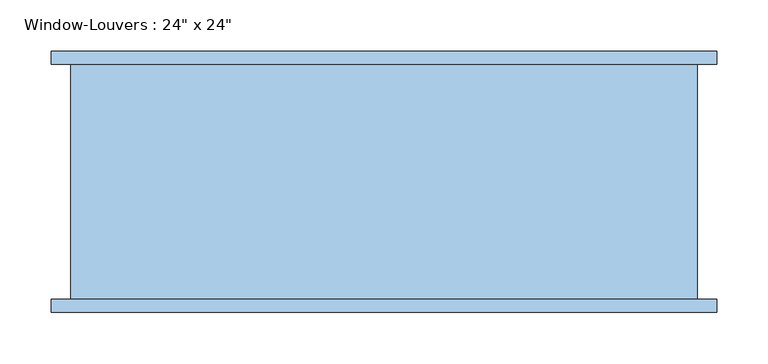
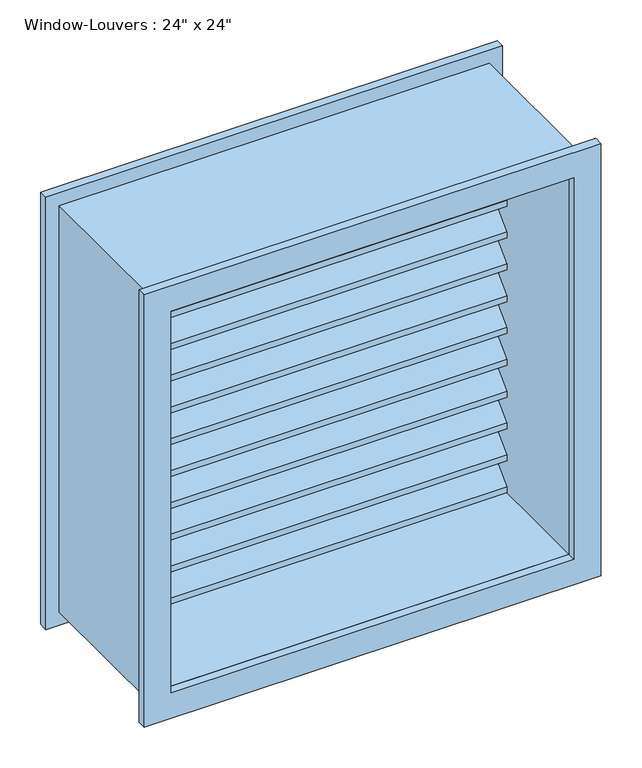
"""IFC4 building model written with IfcOpenShell, lengths in millimetres: window geometry."""

from ifc_helpers import new_model, si_unit, frame, origin, place, context, project, spatial, polyline, outline, extrude, source, transform, mapped, element, save


def window_f2d8fef0(model_context):
    return source(origin(), model_context, "Body", "SweptSolid", [
        extrude(outline(polyline([(107.95, 1419.1754778), (107.95, 1410.1952217), (69.85, 1448.2952217), (31.75, 1410.1952217), (31.75, 1419.1754778), (69.85, 1457.2754778), (107.95, 1419.1754778)])), frame((-285.75, 0.0, 0.0), z_axis=(1.0, 0.0, 0.0), x_axis=(0.0, 1.0, 0.0)), (0.0, 0.0, 1.0), 571.5),
        extrude(outline(polyline([(107.95, 1371.5009557), (107.95, 1362.5206995), (69.85, 1400.6206995), (31.75, 1362.5206995), (31.75, 1371.5009557), (69.85, 1409.6009557), (107.95, 1371.5009557)])), frame((-285.75, 0.0, 0.0), z_axis=(1.0, 0.0, 0.0), x_axis=(0.0, 1.0, 0.0)), (0.0, 0.0, 1.0), 571.5),
        extrude(outline(polyline([(107.95, 1323.8264335), (107.95, 1314.8461774), (69.85, 1352.9461774), (31.75, 1314.8461774), (31.75, 1323.8264335), (69.85, 1361.9264335), (107.95, 1323.8264335)])), frame((-285.75, 0.0, 0.0), z_axis=(1.0, 0.0, 0.0), x_axis=(0.0, 1.0, 0.0)), (0.0, 0.0, 1.0), 571.5),
        extrude(outline(polyline([(107.95, 1276.1519113), (107.95, 1267.1716552), (69.85, 1305.2716552), (31.75, 1267.1716552), (31.75, 1276.1519113), (69.85, 1314.2519113), (107.95, 1276.1519113)])), frame((-285.75, 0.0, 0.0), z_axis=(1.0, 0.0, 0.0), x_axis=(0.0, 1.0, 0.0)), (0.0, 0.0, 1.0), 571.5),
        extrude(outline(polyline([(107.95, 1228.4773891), (107.95, 1219.497133), (69.85, 1257.597133), (31.75, 1219.497133), (31.75, 1228.4773891), (69.85, 1266.5773891), (107.95, 1228.4773891)])), frame((-285.75, 0.0, 0.0), z_axis=(1.0, 0.0, 0.0), x_axis=(0.0, 1.0, 0.0)), (0.0, 0.0, 1.0), 571.5),
        extrude(outline(polyline([(107.95, 1180.802867), (107.95, 1171.8226109), (69.85, 1209.9226109), (31.75, 1171.8226109), (31.75, 1180.802867), (69.85, 1218.902867), (107.95, 1180.802867)])), frame((-285.75, 0.0, 0.0), z_axis=(1.0, 0.0, 0.0), x_axis=(0.0, 1.0, 0.0)), (0.0, 0.0, 1.0), 571.5),
        extrude(outline(polyline([(107.95, 1133.1283448), (107.95, 1124.1480887), (69.85, 1162.2480887), (31.75, 1124.1480887), (31.75, 1133.1283448), (69.85, 1171.2283448), (107.95, 1133.1283448)])), frame((-285.75, 0.0, 0.0), z_axis=(1.0, 0.0, 0.0), x_axis=(0.0, 1.0, 0.0)), (0.0, 0.0, 1.0), 571.5),
        extrude(outline(polyline([(107.95, 1085.4538226), (107.95, 1076.4735665), (69.85, 1114.5735665), (31.75, 1076.4735665), (31.75, 1085.4538226), (69.85, 1123.5538226), (107.95, 1085.4538226)])), frame((-285.75, 0.0, 0.0), z_axis=(1.0, 0.0, 0.0), x_axis=(0.0, 1.0, 0.0)), (0.0, 0.0, 1.0), 571.5),
        extrude(outline(polyline([(107.95, 1037.7793005), (107.95, 1028.7990443), (69.85, 1066.8990443), (31.75, 1028.7990443), (31.75, 1037.7793005), (69.85, 1075.8793005), (107.95, 1037.7793005)])), frame((-285.75, 0.0, 0.0), z_axis=(1.0, 0.0, 0.0), x_axis=(0.0, 1.0, 0.0)), (0.0, 0.0, 1.0), 571.5),
        extrude(outline(polyline([(107.95, 990.1047783), (107.95, 981.1245222), (69.85, 1019.2245222), (31.75, 981.1245222), (31.75, 990.1047783), (69.85, 1028.2047783), (107.95, 990.1047783)])), frame((-285.75, 0.0, 0.0), z_axis=(1.0, 0.0, 0.0), x_axis=(0.0, 1.0, 0.0)), (0.0, 0.0, 1.0), 571.5),
        extrude(outline(polyline([(107.95, 1466.85), (107.95, 1457.8697439), (69.85, 1495.9697439), (31.75, 1457.8697439), (31.75, 1466.85), (69.85, 1504.95), (107.95, 1466.85)])), frame((-285.75, 0.0, 0.0), z_axis=(1.0, 0.0, 0.0), x_axis=(0.0, 1.0, 0.0)), (0.0, 0.0, 1.0), 571.5),
        extrude(outline(polyline([(107.95, 942.4302561), (107.95, 933.45), (69.85, 971.55), (31.75, 933.45), (31.75, 942.4302561), (69.85, 980.5302561), (107.95, 942.4302561)])), frame((-285.75, 0.0, 0.0), z_axis=(1.0, 0.0, 0.0), x_axis=(0.0, 1.0, 0.0)), (0.0, 0.0, 1.0), 571.5),
        extrude(outline(polyline([(1524.0, 304.8), (1524.0, -304.8), (914.4, -304.8), (914.4, 304.8), (1524.0, 304.8)]), holes=[polyline([(1504.95, 285.75), (933.45, 285.75), (933.45, -285.75), (1504.95, -285.75), (1504.95, 285.75)])]), frame((0.0, -120.65, 0.0), z_axis=(0.0, 1.0, 0.0), x_axis=(0.0, 0.0, 1.0)), (0.0, 0.0, 1.0), 228.6),
        extrude(outline(polyline([(1543.05, 323.85), (1543.05, -323.85), (895.35, -323.85), (895.35, 323.85), (1543.05, 323.85)]), holes=[polyline([(1504.95, 285.75), (933.45, 285.75), (933.45, -285.75), (1504.95, -285.75), (1504.95, 285.75)])]), frame((0.0, -133.35, 0.0), z_axis=(0.0, 1.0, 0.0), x_axis=(0.0, 0.0, 1.0)), (0.0, 0.0, 1.0), 12.7),
        extrude(outline(polyline([(1543.05, -323.85), (895.35, -323.85), (895.35, 323.85), (1543.05, 323.85), (1543.05, -323.85)]), holes=[polyline([(1504.95, -285.75), (1504.95, 285.75), (933.45, 285.75), (933.45, -285.75), (1504.95, -285.75)])]), frame((0.0, 107.95, 0.0), z_axis=(0.0, 1.0, 0.0), x_axis=(0.0, 0.0, 1.0)), (0.0, 0.0, 1.0), 12.7),
    ])


if __name__ == "__main__":
    model = new_model("IFC4")
    model_context = context("Model", 3, world=origin())
    ifc_project = project(units=[si_unit("LENGTHUNIT", "METRE", prefix="MILLI")], contexts=[model_context])
    site = spatial("IfcSite", under=ifc_project)
    building = spatial("IfcBuilding", under=site)
    placement = place(None, origin())
    window_shape = window_f2d8fef0(model_context)
    element("IfcWindow", 1, ObjectType="Window-Louvers : 24\" x 24\"", at=placement, inside=building, context=model_context, shape_type="MappedRepresentation", body=[
        mapped(window_shape, transform((0.0, 0.0, 0.0), x_axis=(1.0, 0.0, 0.0), y_axis=(0.0, 1.0, 0.0), z_axis=(0.0, 0.0, 1.0))),
    ])
    save(model, "model.ifc")

# Revit data of these elements
# Type "Window-Louvers : 24\" x 24\""
#   Type Mark = "19"
#   Construction Type Id = "GSP4R"
#   Assembly Code = "B20"
#   Analytic Construction = "1/8 in Pilkington single glazing"
#   Visual Light Transmittance = 0.9
#   Thermal Resistance (R) = 1.53941 (h·ft²·°F)/BTU
#   Solar Heat Gain Coefficient = 0.78
#   Max Height = 1' - 11.74264"
#   Height = 2' - 0"
#   Heat Transfer Coefficient (U) = 0.6496 BTU/(h·ft²·°F)
#   Blade Width [instance default] = 1' - 10 1/2"
#   Blade Vertical Thickness = 0' - 0.35355"
#   Blade Thickness = 0' - 0 1/4"
#   Blade Spacing = 0' - 1 1/2"
#   Blade Height = 0' - 1.85355"
#   Blade Depth = 0' - 3"
#   Blade Angle = 45.00°
#   Default Sill Height = 3' - 0"
#   Trim Projection_Exterior = 0' - 0 1/2"
#   Trim Projection_Interior = 0' - 0 1/2"
#   Trim Width_Exterior = 0' - 1 1/2"
#   Trim Width_Interior = 0' - 1 1/2"
#   Width = 2' - 0"
#   Max Blade Count = 12
#   Define Thermal Properties by = 1
#   Blade Count = 12
#   Frame Material = Birch
#   Louver Material = Birch
#   Trim Exterior Material = Birch
#   Trim Interior Material = Birch
#   Wall Closure = (empty or 0)
# Element 1 (IfcWindow, "Window-Louvers : 24\" x 24\"")
#   Materials on its faces: "Birch"
# Materials
#   "Birch": class "Wood", colour RGB 224 178 126, transparency 0, Description = "Betula Alleghaniensis", Cost = 0
